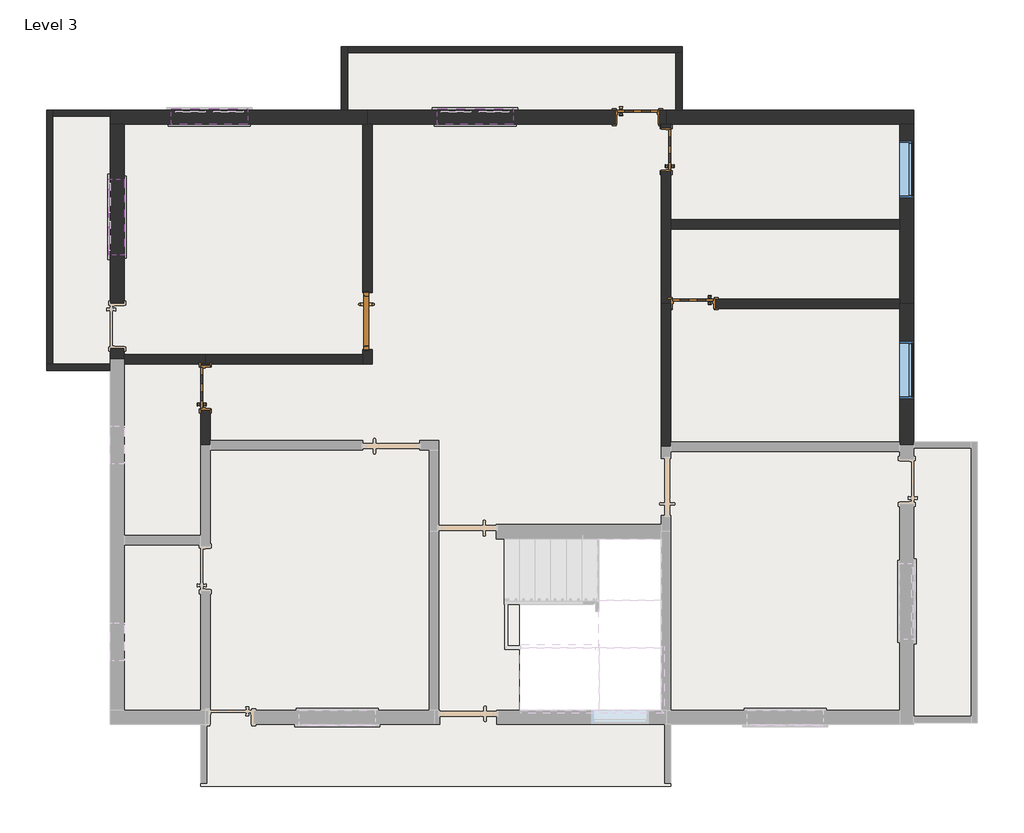
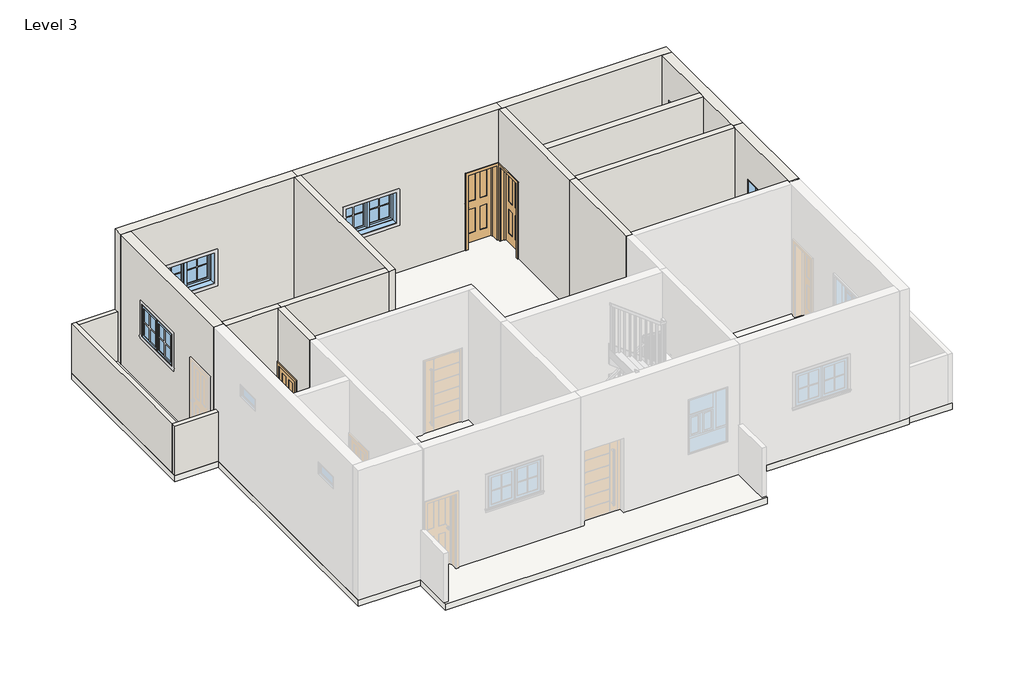
# One storey, part 2 of 3: 20 walls, 5 doors, 5 windows, 1 slab.
"""IFC4 building model written with IfcOpenShell, lengths in millimetres."""

from ifc_helpers import new_model, si_unit, frame, origin, place, context, project, spatial, polyline, outline, extrude, faceted_brep, transform, mapped, element, save
from components import door_3_44036f4b, door_a03dd1d4, door_7109d6db, door_46909e31, m_window_awning_double_horizontal_4_8afcb0b2, m_window_casement_double_sash_variable_3_661e274a

model = new_model("IFC4")

# Units and contexts
model_context = context("Model", 3, world=origin())
ifc_project = project(units=[si_unit("LENGTHUNIT", "METRE", prefix="MILLI")], contexts=[model_context])

# Site, building, storey
site = spatial("IfcSite", under=ifc_project)
building = spatial("IfcBuilding", under=site)
storey = spatial("IfcBuildingStorey", under=building, Name="Level 3", Elevation=6400.8)

# Doors
placement = place(None, origin())
door_3_shape = door_3_44036f4b(model_context)
element("IfcDoor", 1, ObjectType="3'", at=placement, inside=storey, context=model_context, shape_type="MappedRepresentation", body=[
    mapped(door_3_shape, transform((-14176.5794909, 1971.8381491, 6400.8), x_axis=(0.0, -1.0, 0.0), y_axis=(1.0, 0.0, 0.0), z_axis=(0.0, 0.0, 1.0))),
])
door_shape = door_a03dd1d4(model_context)
element("IfcDoor", 2, ObjectType="M_Door-Interior-Single-4_Panel-Wood : 2'2\"", at=placement, inside=storey, context=model_context, shape_type="MappedRepresentation", body=[
    mapped(door_shape, transform((-16770.5544909, 905.4381491, 6400.8), x_axis=(0.0, 1.0, 0.0), y_axis=(-1.0, 0.0, 0.0), z_axis=(0.0, 0.0, 1.0))),
])
door_2_shape = door_7109d6db(model_context)
element("IfcDoor", 3, ObjectType="M_Door-Interior-Single-4_Panel-Wood : 2'2\"", at=placement, inside=storey, context=model_context, shape_type="MappedRepresentation", body=[
    mapped(door_2_shape, transform((-9398.2044909, 4715.4381491, 6400.8), x_axis=(0.0, 1.0, 0.0), y_axis=(-1.0, 0.0, 0.0), z_axis=(0.0, 0.0, 1.0))),
])
element("IfcDoor", 4, ObjectType="M_Door-Interior-Single-4_Panel-Wood : 2'2\"", at=placement, inside=storey, context=model_context, shape_type="MappedRepresentation", body=[
    mapped(door_2_shape, transform((-8969.9794909, 2254.4131491, 6400.8), x_axis=(-1.0, 0.0, 0.0), y_axis=(0.0, -1.0, 0.0), z_axis=(0.0, 0.0, 1.0))),
])
door_4_shape = door_46909e31(model_context)
element("IfcDoor", 5, ObjectType="M_Door-Interior-Single-4_Panel-Wood : 2'2\"", at=placement, inside=storey, context=model_context, shape_type="MappedRepresentation", body=[
    mapped(door_4_shape, transform((-9858.1794909, 5238.9131491, 6400.8), x_axis=(1.0, 0.0, 0.0), y_axis=(0.0, 1.0, 0.0), z_axis=(0.0, 0.0, 1.0))),
])

# Slab
element("IfcSlab", 6, ObjectType="Generic 150mm", at=placement, inside=storey, context=model_context, shape_type="SweptSolid", body=[
    extrude(outline(polyline([(-18291.3794909, 1184.4381491), (-19307.3794909, 1184.4381491), (-19307.3794909, 5350.0381491), (-14596.2721539, 5350.0381491), (-14596.2721539, 6366.0381491), (-9142.3367869, 6366.0381491), (-9142.3367869, 5350.0381491), (-5438.9794909, 5350.0381491), (-5438.9794909, 41.4381491), (-4422.9794909, 41.4381491), (-4422.9794909, -4454.3618509), (-5438.9794909, -4454.3618509), (-5438.9794909, -4479.7618509), (-9325.1794909, -4479.7618509), (-9325.1794909, -5470.3618509), (-16843.5794909, -5470.3618509), (-16843.5794909, -4479.7618509), (-18291.3794909, -4479.7618509), (-18291.3794909, 1184.4381491)]), holes=[polyline([(-11738.1794909, -1507.9618509), (-11738.1794909, -4251.1618509), (-9477.5794909, -4251.1618509), (-9477.5794909, -1507.9618509), (-11738.1794909, -1507.9618509)])]), frame((0.0, 0.0, 6250.8), z_axis=(0.0, 0.0, 1.0), x_axis=(1.0, 0.0, 0.0)), (0.0, 0.0, 1.0), 150.0),
])

# Walls
element("IfcWall", 7, ObjectType="Generic - 4\"", at=placement, inside=storey, context=model_context, shape_type="Brep", body=[
    faceted_brep([(-14494.6721539, 5350.0381491, 6400.8), (-14494.6721539, 6264.4381491, 6400.8), (-14494.6721539, 6366.0381491, 6400.8), (-14494.6721539, 6366.0381491, 7620.0), (-14494.6721539, 6264.4381491, 7620.0), (-14494.6721539, 5350.0381491, 7620.0), (-14596.2721539, 5350.0381491, 6400.8), (-14596.2721539, 5350.0381491, 7620.0), (-14596.2721539, 6366.0381491, 7620.0), (-14596.2721539, 6366.0381491, 6400.8)], [[[0, 1, 2, 3, 4, 5]], [[6, 7, 8, 9]], [[2, 1, 0, 6, 9]], [[5, 4, 3, 8, 7]], [[0, 5, 7, 6]], [[3, 2, 9, 8]]]),
])
element("IfcWall", 8, ObjectType="Generic - 4\"", at=placement, inside=storey, context=model_context, shape_type="Brep", body=[
    faceted_brep([(-14494.6721539, 6264.4381491, 6400.8), (-9243.9367869, 6264.4381491, 6400.8), (-9142.3367869, 6264.4381491, 6400.8), (-9142.3367869, 6264.4381491, 7620.0), (-9243.9367869, 6264.4381491, 7620.0), (-14494.6721539, 6264.4381491, 7620.0), (-14494.6721539, 6366.0381491, 6400.8), (-14494.6721539, 6366.0381491, 7620.0), (-9142.3367869, 6366.0381491, 7620.0), (-9142.3367869, 6366.0381491, 6400.8)], [[[0, 1, 2, 3, 4, 5]], [[6, 7, 8, 9]], [[2, 1, 0, 6, 9]], [[5, 4, 3, 8, 7]], [[0, 5, 7, 6]], [[3, 2, 9, 8]]]),
])
element("IfcWall", 9, ObjectType="Generic - 4\"", at=placement, inside=storey, context=model_context, shape_type="SweptSolid", body=[
    extrude(outline(polyline([(-9243.9367869, 5350.0381491), (-9243.9367869, 6264.4381491), (-9142.3367869, 6264.4381491), (-9142.3367869, 5350.0381491), (-9243.9367869, 5350.0381491)])), frame((0.0, 0.0, 6400.8), z_axis=(0.0, 0.0, 1.0), x_axis=(1.0, 0.0, 0.0)), (0.0, 0.0, 1.0), 1219.2),
])
element("IfcWall", 10, ObjectType="Generic - 4\"", at=placement, inside=storey, context=model_context, shape_type="Brep", body=[
    faceted_brep([(-19307.3794909, 1184.4381491, 6400.8), (-18291.3794909, 1184.4381491, 6400.8), (-18291.3794909, 1184.4381491, 7620.0), (-19307.3794909, 1184.4381491, 7620.0), (-19307.3794909, 1286.0381491, 6400.8), (-19307.3794909, 1286.0381491, 7620.0), (-19205.7794909, 1286.0381491, 7620.0), (-18291.3794909, 1286.0381491, 7620.0), (-18291.3794909, 1286.0381491, 6400.8), (-19205.7794909, 1286.0381491, 6400.8)], [[[0, 1, 2, 3]], [[4, 5, 6, 7, 8, 9]], [[1, 0, 4, 9, 8]], [[3, 2, 7, 6, 5]], [[2, 1, 8, 7]], [[0, 3, 5, 4]]]),
])
element("IfcWall", 11, ObjectType="Generic - 4\"", at=placement, inside=storey, context=model_context, shape_type="Brep", body=[
    faceted_brep([(-19307.3794909, 5350.0381491, 6400.8), (-19307.3794909, 1286.0381491, 6400.8), (-19307.3794909, 1286.0381491, 7620.0), (-19307.3794909, 5350.0381491, 7620.0), (-19205.7794909, 5350.0381491, 6400.8), (-19205.7794909, 5350.0381491, 7620.0), (-19205.7794909, 5248.4381491, 7620.0), (-19205.7794909, 1286.0381491, 7620.0), (-19205.7794909, 1286.0381491, 6400.8), (-19205.7794909, 5248.4381491, 6400.8)], [[[0, 1, 2, 3]], [[4, 5, 6, 7, 8, 9]], [[1, 0, 4, 9, 8]], [[3, 2, 7, 6, 5]], [[2, 1, 8, 7]], [[0, 3, 5, 4]]]),
])
element("IfcWall", 12, ObjectType="Generic - 4\"", at=placement, inside=storey, context=model_context, shape_type="SweptSolid", body=[
    extrude(outline(polyline([(-19205.7794909, 5350.0381491), (-18291.3794909, 5350.0381491), (-18291.3794909, 5248.4381491), (-19205.7794909, 5248.4381491), (-19205.7794909, 5350.0381491)])), frame((0.0, 0.0, 6400.8), z_axis=(0.0, 0.0, 1.0), x_axis=(1.0, 0.0, 0.0)), (0.0, 0.0, 1.0), 1219.2),
])
element("IfcWall", 13, ObjectType="Generic - 6\"", at=placement, inside=storey, context=model_context, shape_type="Brep", body=[
    faceted_brep([(-14252.7794909, 1286.0381491, 9601.2), (-14252.7794909, 1438.4381491, 9601.2), (-14252.7794909, 5121.4381491, 9601.2), (-14252.7794909, 5121.4381491, 6400.8), (-14252.7794909, 2429.0381491, 6400.8), (-14252.7794909, 2429.0381491, 8229.6), (-14252.7794909, 1514.6381491, 8229.6), (-14252.7794909, 1514.6381491, 6400.8), (-14252.7794909, 1438.4381491, 6400.8), (-14252.7794909, 1286.0381491, 6400.8), (-14100.3794909, 5121.4381491, 9601.2), (-14100.3794909, 1286.0381491, 9601.2), (-14100.3794909, 1286.0381491, 6400.8), (-14100.3794909, 1514.6381491, 6400.8), (-14100.3794909, 1514.6381491, 8229.6), (-14100.3794909, 2429.0381491, 8229.6), (-14100.3794909, 2429.0381491, 6400.8), (-14100.3794909, 5121.4381491, 6400.8), (-14232.7794909, 1514.6381491, 6400.8), (-14232.7794909, 1499.6381491, 6400.8), (-14155.7794909, 1499.6381491, 6400.8), (-14155.7794909, 1514.6381491, 6400.8), (-14176.5794909, 5121.4381491, 6400.8), (-14155.7794909, 2429.0381491, 6400.8), (-14155.7794909, 2444.0381491, 6400.8), (-14232.7794909, 2444.0381491, 6400.8), (-14232.7794909, 2429.0381491, 6400.8), (-14176.5794909, 5121.4381491, 9601.2), (-14232.7794909, 2429.0381491, 8229.6), (-14232.7794909, 1514.6381491, 8229.6), (-14155.7794909, 1514.6381491, 8229.6), (-14155.7794909, 2429.0381491, 8229.6), (-14232.7794909, 2444.0381491, 8244.6), (-14155.7794909, 2444.0381491, 8244.6), (-14155.7794909, 1499.6381491, 8244.6), (-14232.7794909, 1499.6381491, 8244.6)], [[[0, 1, 2, 3, 4, 5, 6, 7, 8, 9]], [[10, 11, 12, 13, 14, 15, 16, 17]], [[12, 9, 8, 7, 18, 19, 20, 21, 13]], [[3, 22, 17, 16, 23, 24, 25, 26, 4]], [[2, 1, 0, 11, 10, 27]], [[3, 2, 27, 10, 17, 22]], [[0, 9, 12, 11]], [[5, 28, 29, 6]], [[14, 30, 31, 15]], [[6, 29, 18, 7]], [[30, 14, 13, 21]], [[28, 5, 4, 26]], [[15, 31, 23, 16]], [[32, 33, 34, 35]], [[35, 34, 20, 19]], [[31, 30, 21, 20, 34, 33, 24, 23]], [[33, 32, 25, 24]], [[29, 28, 26, 25, 32, 35, 19, 18]]]),
])
element("IfcWall", 14, ObjectType="Generic - 6\"", at=placement, inside=storey, context=model_context, shape_type="Brep", body=[
    faceted_brep([(-14252.7794909, 1438.4381491, 6400.8), (-16767.3794909, 1438.4381491, 6400.8), (-16767.3794909, 1438.4381491, 9601.2), (-14252.7794909, 1438.4381491, 9601.2), (-14252.7794909, 1286.0381491, 6400.8), (-14252.7794909, 1286.0381491, 9601.2), (-16691.1794909, 1286.0381491, 9601.2), (-16767.3794909, 1286.0381491, 9601.2), (-16767.3794909, 1286.0381491, 6400.8), (-16691.1794909, 1286.0381491, 6400.8)], [[[0, 1, 2, 3]], [[4, 5, 6, 7, 8, 9]], [[1, 0, 4, 9, 8]], [[2, 1, 8, 7]], [[3, 2, 7, 6, 5]], [[0, 3, 5, 4]]]),
])
element("IfcWall", 15, ObjectType="Generic - 6\"", at=placement, inside=storey, context=model_context, shape_type="SweptSolid", body=[
    extrude(outline(polyline([(-5667.5794909, 3445.0381491), (-9325.1794909, 3445.0381491), (-9325.1794909, 3597.4381491), (-5667.5794909, 3597.4381491), (-5667.5794909, 3445.0381491)])), frame((0.0, 0.0, 6400.8), z_axis=(0.0, 0.0, 1.0), x_axis=(1.0, 0.0, 0.0)), (0.0, 0.0, 1.0), 3200.4),
])
element("IfcWall", 16, ObjectType="Generic - 6\"", at=placement, inside=storey, context=model_context, shape_type="Brep", body=[
    faceted_brep([(-9325.1794909, 2327.4381491, 9601.2), (-5667.5794909, 2327.4381491, 9601.2), (-5667.5794909, 2327.4381491, 6400.8), (-8614.7794909, 2327.4381491, 6400.8), (-8614.7794909, 2327.4381491, 8254.6), (-9325.1794909, 2327.4381491, 8254.6), (-5667.5794909, 2175.0381491, 9601.2), (-9325.1794909, 2175.0381491, 9601.2), (-9325.1794909, 2175.0381491, 8254.6), (-8614.7794909, 2175.0381491, 8254.6), (-8614.7794909, 2175.0381491, 6400.8), (-5667.5794909, 2175.0381491, 6400.8), (-5667.5794909, 2251.2381491, 6400.8), (-9325.1794909, 2251.2381491, 9601.2), (-5667.5794909, 2251.2381491, 9601.2)], [[[0, 1, 2, 3, 4, 5]], [[6, 7, 8, 9, 10, 11]], [[2, 12, 11, 10, 3]], [[1, 0, 13, 7, 6, 14]], [[2, 1, 14, 6, 11, 12]], [[7, 13, 0, 5, 8]], [[4, 9, 8, 5]], [[9, 4, 3, 10]]]),
])
element("IfcWall", 17, ObjectType="Generic - 6\"", at=placement, inside=storey, context=model_context, shape_type="Brep", body=[
    faceted_brep([(-9325.1794909, 5121.4381491, 9601.2), (-9325.1794909, 3597.4381491, 9601.2), (-9325.1794909, 3445.0381491, 9601.2), (-9325.1794909, 2327.4381491, 9601.2), (-9325.1794909, 2251.2381491, 9601.2), (-9325.1794909, 2251.2381491, 6400.8), (-9325.1794909, 3445.0381491, 6400.8), (-9325.1794909, 3597.4381491, 6400.8), (-9325.1794909, 4360.2381491, 6400.8), (-9325.1794909, 4360.2381491, 8254.6), (-9325.1794909, 5070.6381491, 8254.6), (-9325.1794909, 5070.6381491, 6400.8), (-9325.1794909, 5121.4381491, 6400.8), (-9477.5794909, 2251.2381491, 9601.2), (-9477.5794909, 5121.4381491, 9601.2), (-9477.5794909, 5121.4381491, 6400.8), (-9477.5794909, 5070.6381491, 6400.8), (-9477.5794909, 5070.6381491, 8254.6), (-9477.5794909, 4360.2381491, 8254.6), (-9477.5794909, 4360.2381491, 6400.8), (-9477.5794909, 2251.2381491, 6400.8), (-9401.3794909, 5121.4381491, 6400.8), (-9401.3794909, 5121.4381491, 9601.2)], [[[0, 1, 2, 3, 4, 5, 6, 7, 8, 9, 10, 11, 12]], [[13, 14, 15, 16, 17, 18, 19, 20]], [[15, 21, 12, 11, 16]], [[5, 20, 19, 8, 7, 6]], [[4, 3, 2, 1, 0, 22, 14, 13]], [[5, 4, 13, 20]], [[0, 12, 21, 15, 14, 22]], [[10, 17, 16, 11]], [[17, 10, 9, 18]], [[18, 9, 8, 19]]]),
])
element("IfcWall", 18, ObjectType="Generic - 6\"", at=placement, inside=storey, context=model_context, shape_type="Brep", body=[
    faceted_brep([(-9325.1794909, -34.7618509, 6400.8), (-9325.1794909, 41.4381491, 6400.8), (-9325.1794909, 2251.2381491, 6400.8), (-9325.1794909, 2251.2381491, 9601.2), (-9325.1794909, 2175.0381491, 9601.2), (-9325.1794909, 41.4381491, 9601.2), (-9325.1794909, -34.7618509, 9601.2), (-9477.5794909, -34.7618509, 6400.8), (-9477.5794909, -34.7618509, 9601.2), (-9477.5794909, 2251.2381491, 9601.2), (-9477.5794909, 2251.2381491, 6400.8)], [[[0, 1, 2, 3, 4, 5, 6]], [[7, 8, 9, 10]], [[2, 1, 0, 7, 10]], [[3, 2, 10, 9]], [[6, 5, 4, 3, 9, 8]], [[0, 6, 8, 7]]]),
])
element("IfcWall", 19, ObjectType="Generic - 6\"", at=placement, inside=storey, context=model_context, shape_type="Brep", body=[
    faceted_brep([(-16691.1794909, 1286.0381491, 9601.2), (-16691.1794909, 66.8381491, 9601.2), (-16691.1794909, -9.3618509, 9601.2), (-16691.1794909, -9.3618509, 6400.8), (-16691.1794909, 66.8381491, 6400.8), (-16691.1794909, 550.2381491, 6400.8), (-16691.1794909, 550.2381491, 8254.6), (-16691.1794909, 1260.6381491, 8254.6), (-16691.1794909, 1260.6381491, 6400.8), (-16691.1794909, 1286.0381491, 6400.8), (-16843.5794909, -9.3618509, 9601.2), (-16843.5794909, 1286.0381491, 9601.2), (-16843.5794909, 1286.0381491, 6400.8), (-16843.5794909, 1260.6381491, 6400.8), (-16843.5794909, 1260.6381491, 8254.6), (-16843.5794909, 550.2381491, 8254.6), (-16843.5794909, 550.2381491, 6400.8), (-16843.5794909, -9.3618509, 6400.8), (-16767.3794909, 1286.0381491, 6400.8), (-16767.3794909, 1286.0381491, 9601.2)], [[[0, 1, 2, 3, 4, 5, 6, 7, 8, 9]], [[10, 11, 12, 13, 14, 15, 16, 17]], [[12, 18, 9, 8, 13]], [[3, 17, 16, 5, 4]], [[2, 1, 0, 19, 11, 10]], [[3, 2, 10, 17]], [[0, 9, 18, 12, 11, 19]], [[7, 14, 13, 8]], [[14, 7, 6, 15]], [[15, 6, 5, 16]]]),
])
element("IfcWall", 20, ObjectType="Generic - 6\"", at=placement, inside=storey, context=model_context, shape_type="Brep", body=[
    faceted_brep([(-16767.3794909, 1438.4381491, 6400.8), (-18062.7794909, 1438.4381491, 6400.8), (-18062.7794909, 1438.4381491, 9601.2), (-16767.3794909, 1438.4381491, 9601.2), (-16767.3794909, 1286.0381491, 6400.8), (-16767.3794909, 1286.0381491, 9601.2), (-16843.5794909, 1286.0381491, 9601.2), (-18062.7794909, 1286.0381491, 9601.2), (-18062.7794909, 1286.0381491, 6400.8), (-16843.5794909, 1286.0381491, 6400.8), (-18062.7794909, 1362.2381491, 6400.8), (-18062.7794909, 1362.2381491, 9601.2)], [[[0, 1, 2, 3]], [[4, 5, 6, 7, 8, 9]], [[1, 0, 4, 9, 8, 10]], [[3, 2, 11, 7, 6, 5]], [[0, 3, 5, 4]], [[2, 1, 10, 8, 7, 11]]]),
])
element("IfcWall", 21, ObjectType="Generic - 9\"", at=placement, inside=storey, context=model_context, shape_type="Brep", body=[
    faceted_brep([(-18291.3794909, 5121.4381491, 9601.2), (-18291.3794909, 5121.4381491, 6400.8), (-18062.7794909, 5121.4381491, 6400.8), (-14252.7794909, 5121.4381491, 6400.8), (-14176.5794909, 5121.4381491, 6400.8), (-14176.5794909, 5121.4381491, 9601.2), (-14252.7794909, 5121.4381491, 9601.2), (-18062.7794909, 5121.4381491, 9601.2), (-16094.2794909, 5121.4381491, 8420.0), (-16094.2794909, 5121.4381491, 7620.0), (-17313.4794909, 5121.4381491, 7620.0), (-17313.4794909, 5121.4381491, 8420.0), (-18291.3794909, 5350.0381491, 6400.8), (-18291.3794909, 5350.0381491, 9601.2), (-14176.5794909, 5350.0381491, 9601.2), (-14176.5794909, 5350.0381491, 6400.8), (-14494.6721539, 5350.0381491, 6400.8), (-14596.2721539, 5350.0381491, 6400.8), (-16094.2794909, 5350.0381491, 8420.0), (-17313.4794909, 5350.0381491, 8420.0), (-17313.4794909, 5350.0381491, 7620.0), (-16094.2794909, 5350.0381491, 7620.0), (-18291.3794909, 5248.4381491, 6400.8)], [[[0, 1, 2, 3, 4, 5, 6, 7], [8, 9, 10, 11]], [[12, 13, 14, 15, 16, 17], [18, 19, 20, 21]], [[4, 3, 2, 1, 22, 12, 17, 16, 15]], [[5, 4, 15, 14]], [[0, 7, 6, 5, 14, 13]], [[0, 13, 12, 22, 1]], [[9, 8, 18, 21]], [[10, 9, 21, 20]], [[11, 10, 20, 19]], [[8, 11, 19, 18]]]),
])
element("IfcWall", 22, ObjectType="Generic - 9\"", at=placement, inside=storey, context=model_context, shape_type="Brep", body=[
    faceted_brep([(-5667.5794909, 5121.4381491, 6400.8), (-5667.5794909, 3597.4381491, 6400.8), (-5667.5794909, 3445.0381491, 6400.8), (-5667.5794909, 2327.4381491, 6400.8), (-5667.5794909, 2251.2381491, 6400.8), (-5667.5794909, 2251.2381491, 9601.2), (-5667.5794909, 2327.4381491, 9601.2), (-5667.5794909, 3445.0381491, 9601.2), (-5667.5794909, 3597.4381491, 9601.2), (-5667.5794909, 5121.4381491, 9601.2), (-5667.5794909, 3943.5131491, 8650.8), (-5667.5794909, 3943.5131491, 7300.8), (-5667.5794909, 4857.9131491, 7300.8), (-5667.5794909, 4857.9131491, 8650.8), (-5438.9794909, 5121.4381491, 6400.8), (-5438.9794909, 5121.4381491, 9601.2), (-5438.9794909, 2251.2381491, 9601.2), (-5438.9794909, 2251.2381491, 6400.8), (-5438.9794909, 3943.5131491, 8650.8), (-5438.9794909, 4857.9131491, 8650.8), (-5438.9794909, 4857.9131491, 7300.8), (-5438.9794909, 3943.5131491, 7300.8)], [[[0, 1, 2, 3, 4, 5, 6, 7, 8, 9], [10, 11, 12, 13]], [[14, 15, 16, 17], [18, 19, 20, 21]], [[4, 3, 2, 1, 0, 14, 17]], [[5, 4, 17, 16]], [[9, 8, 7, 6, 5, 16, 15]], [[0, 9, 15, 14]], [[11, 10, 18, 21]], [[12, 11, 21, 20]], [[13, 12, 20, 19]], [[10, 13, 19, 18]]]),
])
element("IfcWall", 23, ObjectType="Generic - 9\"", at=placement, inside=storey, context=model_context, shape_type="Brep", body=[
    faceted_brep([(-9401.3794909, 5121.4381491, 6400.8), (-9401.3794909, 5121.4381491, 9601.2), (-9477.5794909, 5121.4381491, 9601.2), (-14100.3794909, 5121.4381491, 9601.2), (-14176.5794909, 5121.4381491, 9601.2), (-14176.5794909, 5121.4381491, 6400.8), (-14100.3794909, 5121.4381491, 6400.8), (-10213.3794909, 5121.4381491, 6400.8), (-10213.3794909, 5121.4381491, 8254.6), (-9502.9794909, 5121.4381491, 8254.6), (-9502.9794909, 5121.4381491, 6400.8), (-9477.5794909, 5121.4381491, 6400.8), (-11844.5419909, 5121.4381491, 8420.0), (-11844.5419909, 5121.4381491, 7620.0), (-13063.7419909, 5121.4381491, 7620.0), (-13063.7419909, 5121.4381491, 8420.0), (-9401.3794909, 5350.0381491, 9601.2), (-9401.3794909, 5350.0381491, 6400.8), (-9502.9794909, 5350.0381491, 6400.8), (-9502.9794909, 5350.0381491, 8254.6), (-10213.3794909, 5350.0381491, 8254.6), (-10213.3794909, 5350.0381491, 6400.8), (-14176.5794909, 5350.0381491, 6400.8), (-14176.5794909, 5350.0381491, 9601.2), (-11844.5419909, 5350.0381491, 8420.0), (-13063.7419909, 5350.0381491, 8420.0), (-13063.7419909, 5350.0381491, 7620.0), (-11844.5419909, 5350.0381491, 7620.0)], [[[0, 1, 2, 3, 4, 5, 6, 7, 8, 9, 10, 11], [12, 13, 14, 15]], [[16, 17, 18, 19, 20, 21, 22, 23], [24, 25, 26, 27]], [[5, 22, 21, 7, 6]], [[17, 0, 11, 10, 18]], [[1, 0, 17, 16]], [[4, 3, 2, 1, 16, 23]], [[5, 4, 23, 22]], [[12, 15, 25, 24]], [[15, 14, 26, 25]], [[14, 13, 27, 26]], [[13, 12, 24, 27]], [[9, 19, 18, 10]], [[19, 9, 8, 20]], [[20, 8, 7, 21]]]),
])
element("IfcWall", 24, ObjectType="Generic - 9\"", at=placement, inside=storey, context=model_context, shape_type="Brep", body=[
    faceted_brep([(-9401.3794909, 5121.4381491, 6400.8), (-9325.1794909, 5121.4381491, 6400.8), (-5667.5794909, 5121.4381491, 6400.8), (-5438.9794909, 5121.4381491, 6400.8), (-5438.9794909, 5121.4381491, 9601.2), (-5667.5794909, 5121.4381491, 9601.2), (-9325.1794909, 5121.4381491, 9601.2), (-9401.3794909, 5121.4381491, 9601.2), (-9401.3794909, 5350.0381491, 6400.8), (-9401.3794909, 5350.0381491, 9601.2), (-5438.9794909, 5350.0381491, 9601.2), (-5438.9794909, 5350.0381491, 6400.8), (-9142.3367869, 5350.0381491, 6400.8), (-9243.9367869, 5350.0381491, 6400.8)], [[[0, 1, 2, 3, 4, 5, 6, 7]], [[8, 9, 10, 11, 12, 13]], [[3, 2, 1, 0, 8, 13, 12, 11]], [[7, 6, 5, 4, 10, 9]], [[0, 7, 9, 8]], [[4, 3, 11, 10]]]),
])
element("IfcWall", 25, ObjectType="Generic - 9\"", at=placement, inside=storey, context=model_context, shape_type="Brep", body=[
    faceted_brep([(-5667.5794909, 2251.2381491, 6400.8), (-5667.5794909, 2175.0381491, 6400.8), (-5667.5794909, 41.4381491, 6400.8), (-5667.5794909, -34.7618509, 6400.8), (-5667.5794909, -34.7618509, 9601.2), (-5667.5794909, 41.4381491, 9601.2), (-5667.5794909, 2175.0381491, 9601.2), (-5667.5794909, 2251.2381491, 9601.2), (-5667.5794909, 732.0006491, 8650.8), (-5667.5794909, 732.0006491, 7300.8), (-5667.5794909, 1646.4006491, 7300.8), (-5667.5794909, 1646.4006491, 8650.8), (-5438.9794909, 2251.2381491, 6400.8), (-5438.9794909, 2251.2381491, 9601.2), (-5438.9794909, -34.7618509, 9601.2), (-5438.9794909, -34.7618509, 6400.8), (-5438.9794909, 41.4381491, 6400.8), (-5438.9794909, 732.0006491, 8650.8), (-5438.9794909, 1646.4006491, 8650.8), (-5438.9794909, 1646.4006491, 7300.8), (-5438.9794909, 732.0006491, 7300.8)], [[[0, 1, 2, 3, 4, 5, 6, 7], [8, 9, 10, 11]], [[12, 13, 14, 15, 16], [17, 18, 19, 20]], [[3, 2, 1, 0, 12, 16, 15]], [[7, 6, 5, 4, 14, 13]], [[0, 7, 13, 12]], [[8, 11, 18, 17]], [[11, 10, 19, 18]], [[10, 9, 20, 19]], [[9, 8, 17, 20]], [[3, 15, 14, 4]]]),
])
element("IfcWall", 26, ObjectType="Generic - 9\"", at=placement, inside=storey, context=model_context, shape_type="Brep", body=[
    faceted_brep([(-18062.7794909, 5121.4381491, 9601.2), (-18062.7794909, 1438.4381491, 9601.2), (-18062.7794909, 1362.2381491, 9601.2), (-18062.7794909, 1362.2381491, 6400.8), (-18062.7794909, 1438.4381491, 6400.8), (-18062.7794909, 1540.0381491, 6400.8), (-18062.7794909, 1540.0381491, 8254.6), (-18062.7794909, 2250.4381491, 8254.6), (-18062.7794909, 2250.4381491, 6400.8), (-18062.7794909, 5121.4381491, 6400.8), (-18062.7794909, 4247.5131491, 8420.0), (-18062.7794909, 4247.5131491, 7620.0), (-18062.7794909, 3028.3131491, 7620.0), (-18062.7794909, 3028.3131491, 8420.0), (-18291.3794909, 1362.2381491, 9601.2), (-18291.3794909, 5121.4381491, 9601.2), (-18291.3794909, 5121.4381491, 6400.8), (-18291.3794909, 2250.4381491, 6400.8), (-18291.3794909, 2250.4381491, 8254.6), (-18291.3794909, 1540.0381491, 8254.6), (-18291.3794909, 1540.0381491, 6400.8), (-18291.3794909, 1362.2381491, 6400.8), (-18291.3794909, 4247.5131491, 8420.0), (-18291.3794909, 3028.3131491, 8420.0), (-18291.3794909, 3028.3131491, 7620.0), (-18291.3794909, 4247.5131491, 7620.0)], [[[0, 1, 2, 3, 4, 5, 6, 7, 8, 9], [10, 11, 12, 13]], [[14, 15, 16, 17, 18, 19, 20, 21], [22, 23, 24, 25]], [[16, 9, 8, 17]], [[3, 21, 20, 5, 4]], [[2, 1, 0, 15, 14]], [[9, 16, 15, 0]], [[10, 13, 23, 22]], [[13, 12, 24, 23]], [[12, 11, 25, 24]], [[11, 10, 22, 25]], [[19, 6, 5, 20]], [[6, 19, 18, 7]], [[7, 18, 17, 8]], [[2, 14, 21, 3]]]),
])

# Windows
m_window_awning_double_horizontal_4_shape = m_window_awning_double_horizontal_4_8afcb0b2(model_context)
element("IfcWindow", 27, ObjectType="M_Window-Awning-Double-Horizontal : 4'", at=placement, inside=storey, context=model_context, shape_type="MappedRepresentation", body=[
    mapped(m_window_awning_double_horizontal_4_shape, transform((-16703.8794909, 5235.7381491, 6720.0), x_axis=(1.0, 0.0, 0.0), y_axis=(0.0, 1.0, 0.0), z_axis=(0.0, 0.0, 1.0))),
])
element("IfcWindow", 28, ObjectType="M_Window-Awning-Double-Horizontal : 4'", at=placement, inside=storey, context=model_context, shape_type="MappedRepresentation", body=[
    mapped(m_window_awning_double_horizontal_4_shape, transform((-18177.0794909, 3637.9131491, 6720.0), x_axis=(0.0, 1.0, 0.0), y_axis=(-1.0, 0.0, 0.0), z_axis=(0.0, 0.0, 1.0))),
])
element("IfcWindow", 29, ObjectType="M_Window-Awning-Double-Horizontal : 4'", at=placement, inside=storey, context=model_context, shape_type="MappedRepresentation", body=[
    mapped(m_window_awning_double_horizontal_4_shape, transform((-12454.1419909, 5235.7381491, 6720.0), x_axis=(1.0, 0.0, 0.0), y_axis=(0.0, 1.0, 0.0), z_axis=(0.0, 0.0, 1.0))),
])
m_window_casement_double_sash_variable_3_shape = m_window_casement_double_sash_variable_3_661e274a(model_context)
element("IfcWindow", 30, ObjectType="M_Window-Casement-Double-Sash-Variable : 3'", at=placement, inside=storey, context=model_context, shape_type="MappedRepresentation", body=[
    mapped(m_window_casement_double_sash_variable_3_shape, transform((-5553.2794909, 1189.2006491, 6400.8), x_axis=(0.0, -1.0, 0.0), y_axis=(1.0, 0.0, 0.0), z_axis=(0.0, 0.0, 1.0))),
])
element("IfcWindow", 31, ObjectType="M_Window-Casement-Double-Sash-Variable : 3'", at=placement, inside=storey, context=model_context, shape_type="MappedRepresentation", body=[
    mapped(m_window_casement_double_sash_variable_3_shape, transform((-5553.2794909, 4400.7131491, 6400.8), x_axis=(0.0, -1.0, 0.0), y_axis=(1.0, 0.0, 0.0), z_axis=(0.0, 0.0, 1.0))),
])

save(model, "model.ifc")

# Revit data of these elements
# Type "3'"
#   Type Mark = "41"
#   Water resistance = "up to Class E900, EN 12208:2001"
#   Uniclass2015Version = "v1.21"
#   Uniclass2015Reference = "Ss_25_30_20_30"
#   Uniclass2015Description = "Frame and door leaf system"
#   URL = "www.aluprof.com"
#   Type IFC Predefined Type = "USERDEFINED"
#   Right-hand / Left-hand door [instance default] = ""
#   Resistance to wind load = "up to Class C5/B5, EN 12210:2001"
#   Insert type = "ST"
#   Hardware [instance default] = ""
#   Product page = "https://aluprof.com/en/architects/offer/window-and-door-systems/panel-doors#visualisation"
#   Operation = "SinglePanelOutwardOpening"
#   Opening type = "Outward"
#   NBSReference = "25-50-20/125"
#   NBSDescription = "Frame and door leaf system"
#   Important = "The actual acceptable construction dimensions are dependent on the selection of profiles and hardware, glazing type, construction weight and the construction’s operating conditions. These should be determined by a suitably qualified person, and using ALUPROF’s calculation software"
#   IfcExportType = "USERDEFINED"
#   IfcExportAs = "IfcDoorType"
#   Handle type [instance default] = ""
#   Manufacturer = "ALUPROF SA"
#   Export Type to IFC As = "IfcDoorType"
#   Door sill type [instance default] = ""
#   Description = "External single-leaf panel door outward opening"
#   Model = "MB-86 ST Panel Door AD07"
#   Content of the recyclate in the material = "69.2%"
#   COBie.Type.WarrantyDurationParts = ""
#   COBie.Type.Name = ""
#   COBie.Type.Manufacturer = "ALUPROF SA"
#   COBie.Space.Name = ""
#   COBie.Floor.Name = ""
#   COBie.Facility.Name = ""
#   COBie.CreatedOn = ""
#   COBie.Component.WarrantyStartDate = ""
#   COBie.Component.Name = "MB-86 ST Panel Door AD07"
#   Burglar resistance = "RC2"
#   Air permeability = "up to Class 4, EN 12207:2001"
#   Width of the active leaf = 2' - 8.17717"
#   Placement in wall = 0' - 0.7874"
#   Thickness = 0' - 3.0315"
#   Height of the opening sash = 5' - 9.44094"
#   Handle Offset = 3' - 5.33858"
#   Rough Height = 6' - 2.40945"
#   Rough Width = 3' - 1.1811"
#   Height = 6' - 0"
#   Width = 3' - 0"
#   Construction depth = 0' - 3.0315"
#   Clear opening width = 2' - 3.94882"
#   Clear opening height = 5' - 8.47638"
#   Height of the array = 0' - 11.08136"
#   Schedule No. [instance default] = 1
#   Handrail [instance default] = yes
#   IsExternal = yes
#   Handle [instance default] = no
#   Door closer [instance default] = no
#   Function = 1
#   COBie.Type = yes
#   COBie = yes
#   Access control [instance default] = no
#   Panel = element 361060
#   Wall Closure = (empty or 0)
# Type "M_Door-Interior-Single-4_Panel-Wood : 2'2\""
#   Type Mark = "43"
#   Assembly Code = "C1020300"
#   Analytic Construction = "Wooden"
#   Top Rail = 0' - 4.72441"
#   Thickness = 0' - 1.37795"
#   Thermal Resistance (R) = 0.455703 (m²·K)/W
#   Swing Angle [instance default] = 90.00°
#   Stiles = 0' - 4.72441"
#   Rough Width = 2' - 3.9685"
#   Rough Height = 6' - 0.98425"
#   Mullion = 0' - 4.52756"
#   Lock Rail = 0' - 7.87402"
#   Height = 6' - 0"
#   Width = 2' - 2"
#   Heat Transfer Coefficient (U) = 2.19465 W/(m²·K)
#   Bottom Rail = 0' - 9.05512"
#   Trim Material = Cherry
#   Panel Material = Cherry
#   Frame Material = Cherry
#   Door Handle Material = Aluminum
#   Visual Light Transmittance = 0
#   Solar Heat Gain Coefficient = 0
#   Wall Closure = (empty or 0)
#   Function = (empty or 0)
# Type "Generic 150mm"
#   Function = 0
#   Layers, outside or top first: 0' - 5.90551" no material (function 1)
# Type "Generic - 4\""
#   Layers, outside or top first: 0' - 4" no material (function 1)
# Type "Generic - 6\""
#   Layers, outside or top first: 0' - 6" no material (function 1)
# Type "Generic - 9\""
#   Layers, outside or top first: 0' - 9" no material (function 1)
# Type "M_Window-Awning-Double-Horizontal : 4'"
#   Type Mark = "28"
#   Fire Rating = "0.5h"
#   Assembly Code = "B2020100"
#   Analytic Construction = "Double glazing - domestic"
#   Window Inset [instance default] = 0' - 0"
#   Wall Thickness [instance default] = 0' - 5.90551"
#   Interior Wall Closure [instance default] = 0' - 2.15551"
#   Half Width = 2' - 0"
#   Visual Light Transmittance = 0.81
#   Thermal Resistance (R) = 0.319569 (m²·K)/W
#   Solar Heat Gain Coefficient = 0.76
#   Rough Width = 4' - 0.59055"
#   Rough Height = 2' - 8.08661"
#   Height = 2' - 7.49606"
#   Heat Transfer Coefficient (U) = 3.12929 W/(m²·K)
#   Frame Extension [instance default] = 0' - 0 1/4"
#   Exterior Wall Closure [instance default] = 0' - 1 1/4"
#   Extension Jamb [instance default] = 0' - 2.15551"
#   Default Sill Height = 2' - 11.43307"
#   Width = 4' - 0"
#   Muntin Visibility = yes
#   Interior Trim Visibility [instance default] = yes
#   Exterior Trim Visibility [instance default] = yes
#   Extension Jamb Visibility [instance default] = yes
#   Interior Trim Material = Wood - Stained
#   Muntin Pattern = M_Muntin Pattern_2x2 : M_Muntin Pattern_2x2
#   Interior Trim = M_Trim-Window-Interior-Flat : Picture Frame
#   Interior Frame Material = Wood - Stained
#   Glass Panel Material = Glass
#   Exterior Trim Material = Clad - White
#   Exterior Trim = M_Trim-Window-Exterior-Flat : with Sill
#   Exterior Frame Material = Clad - White
#   Wall Closure = (empty or 0)
# Type "M_Window-Casement-Double-Sash-Variable : 3'"
#   Type Mark = "36"
#   Fire Rating = "0.5h"
#   Assembly Code = "B2020100"
#   Analytic Construction = "Double glazing - domestic"
#   Window Inset [instance default] = 0' - 0 5/8"
#   Wall Thickness [instance default] = 0' - 5.90551"
#   Visual Light Transmittance = 0.81
#   Transom Height Ratio = 0.3
#   Transom Height = 1' - 3.94488"
#   Thermal Resistance (R) = 0.319569 (m²·K)/W
#   Solar Heat Gain Coefficient = 0.76
#   Rough Width = 3' - 0.59055"
#   Rough Height = 4' - 5.74016"
#   Opening Window Height = 1' - 9.25984"
#   Heat Transfer Coefficient (U) = 3.12929 W/(m²·K)
#   Height = 4' - 5.14961"
#   Frame Gap 3 [instance default] = 0' - 1.65041"
#   Frame Gap 2 [instance default] = 0' - 0.62598"
#   Frame Gap 1 = 0' - 1 51/128"
#   Window Width = 1' - 0"
#   Default Sill Height = 2' - 11.43307"
#   Width = 3' - 0"
#   Frame Material = Metal - Aluminum
#   Glass Panel Material = Glass
#   Wall Closure = (empty or 0)
# Element 1 (IfcDoor, "3'")
#   Right-hand / Left-hand door = ""
#   Hardware = ""
#   Handle type = ""
#   Door sill type = ""
#   Schedule No. = 1
#   Handrail = yes
#   Handle = no
#   Door closer = no
#   Access control = no
#   Phase Created = New Construction
# Elements 2, 3, 4, 5 (IfcDoor, "M_Door-Interior-Single-4_Panel-Wood : 2'2\"")
#   Swing Angle = 90.00°
#   Phase Created = New Construction
#   Materials on its faces: "Cherry", "Aluminum"
# Element 6 (IfcSlab, "Generic 150mm")
#   Height Offset From Level = 0' - 0"
#   Phase Created = New Construction
#   Materials on its faces: "WALL2", "Default Floor", "FLOORING TILES 1"
# Elements 7, 8, 9, 10 (IfcWall, "Generic - 4\"")
#   Top Offset = 0' - 0"
#   Base Offset = 0' - 0"
#   Unconnected Height = 4' - 0"
#   wall height = 4' - 0"
#   Phase Created = New Construction
#   Base Constraint = Level 3
#   Materials on its faces: "Default Wall", "WALL2"
# Elements 11, 12 (IfcWall, "Generic - 4\"")
#   Top Offset = 0' - 0"
#   Base Offset = 0' - 0"
#   Unconnected Height = 4' - 0"
#   wall height = 4' - 0"
#   Phase Created = New Construction
#   Base Constraint = Level 3
#   Materials on its faces: "WALL2", "Default Wall"
# Element 13 (IfcWall, "Generic - 6\"")
#   Top Offset = 0' - 0"
#   Base Offset = 0' - 0"
#   Unconnected Height = 10' - 6"
#   wall height = 10' - 6"
#   Phase Created = New Construction
#   Base Constraint = Level 3
#   Materials on its faces: "Default Wall", "LIVING 2", "BED ROOM WALL1"
# Element 14 (IfcWall, "Generic - 6\"")
#   Top Offset = 0' - 0"
#   Base Offset = 0' - 0"
#   Unconnected Height = 10' - 6"
#   wall height = 10' - 6"
#   Phase Created = New Construction
#   Base Constraint = Level 3
#   Materials on its faces: "Default Wall", "BED ROOM WALL 2", "LIVING 2"
# Element 15 (IfcWall, "Generic - 6\"")
#   Top Offset = 0' - 0"
#   Base Offset = 0' - 0"
#   Unconnected Height = 10' - 6"
#   wall height = 10' - 6"
#   Phase Created = New Construction
#   Base Constraint = Level 3
#   Materials on its faces: "Default Wall", "BED ROOM WALL 3", "BED ROOM WALL1"
# Elements 16, 17 (IfcWall, "Generic - 6\"")
#   Top Offset = 0' - 0"
#   Base Offset = 0' - 0"
#   Unconnected Height = 10' - 6"
#   wall height = 10' - 6"
#   Phase Created = New Construction
#   Base Constraint = Level 3
#   Materials on its faces: "Default Wall", "BED ROOM WALL1", "LIVING 2"
# Element 18 (IfcWall, "Generic - 6\"")
#   Top Offset = 0' - 0"
#   Base Offset = 0' - 0"
#   Unconnected Height = 10' - 6"
#   wall height = 10' - 6"
#   Phase Created = New Construction
#   Base Constraint = Level 3
#   Materials on its faces: "Default Wall", "LIVING", "LIVING 2"
# Element 19 (IfcWall, "Generic - 6\"")
#   Top Offset = 0' - 0"
#   Base Offset = 0' - 0"
#   Unconnected Height = 10' - 6"
#   wall height = 10' - 6"
#   Phase Created = New Construction
#   Base Constraint = Level 3
#   Materials on its faces: "Default Wall", "LIVING 2", "BATH ROOM WALL 1"
# Element 20 (IfcWall, "Generic - 6\"")
#   Top Offset = 0' - 0"
#   Base Offset = 0' - 0"
#   Unconnected Height = 10' - 6"
#   wall height = 10' - 6"
#   Phase Created = New Construction
#   Base Constraint = Level 3
#   Materials on its faces: "Default Wall", "BED ROOM WALL 2", "BATH ROOM WALL 1"
# Element 21 (IfcWall, "Generic - 9\"")
#   Top Offset = 0' - 0"
#   Base Offset = 0' - 0"
#   Unconnected Height = 10' - 6"
#   wall height = 10' - 6"
#   Phase Created = New Construction
#   Base Constraint = Level 3
#   Materials on its faces: "Default Wall", "WALL2", "BED ROOM WALL1"
# Element 22 (IfcWall, "Generic - 9\"")
#   Top Offset = 0' - 0"
#   Base Offset = 0' - 0"
#   Unconnected Height = 10' - 6"
#   wall height = 10' - 6"
#   Phase Created = New Construction
#   Base Constraint = Level 3
#   Materials on its faces: "Default Wall", "BED ROOM WALL 3", "WALL2"
# Elements 23, 25 (IfcWall, "Generic - 9\"")
#   Top Offset = 0' - 0"
#   Base Offset = 0' - 0"
#   Unconnected Height = 10' - 6"
#   wall height = 10' - 6"
#   Phase Created = New Construction
#   Base Constraint = Level 3
#   Materials on its faces: "Default Wall", "LIVING 2", "WALL2"
# Element 24 (IfcWall, "Generic - 9\"")
#   Top Offset = 0' - 0"
#   Base Offset = 0' - 0"
#   Unconnected Height = 10' - 6"
#   wall height = 10' - 6"
#   Phase Created = New Construction
#   Base Constraint = Level 3
#   Materials on its faces: "Default Wall", "WALL2", "BED ROOM WALL 3"
# Element 26 (IfcWall, "Generic - 9\"")
#   Top Offset = 0' - 0"
#   Base Offset = 0' - 0"
#   Unconnected Height = 10' - 6"
#   wall height = 10' - 6"
#   Phase Created = New Construction
#   Base Constraint = Level 3
#   Materials on its faces: "Default Wall", "BED ROOM WALL 2", "WALL2"
# Element 27 (IfcWindow, "M_Window-Awning-Double-Horizontal : 4'")
#   Mark = "24"
#   Window Inset = 0' - 0"
#   Interior Wall Closure = 0' - 2.15551"
#   Frame Extension = 0' - 0 1/4"
#   Exterior Wall Closure = 0' - 1 1/4"
#   Interior Trim Visibility = yes
#   Exterior Trim Visibility = yes
#   Phase Created = New Construction
#   Materials on its faces: "Wood - Stained", "Glass", "Clad - White"
# Element 28 (IfcWindow, "M_Window-Awning-Double-Horizontal : 4'")
#   Mark = "25"
#   Window Inset = 0' - 0"
#   Interior Wall Closure = 0' - 2.15551"
#   Frame Extension = 0' - 0 1/4"
#   Exterior Wall Closure = 0' - 1 1/4"
#   Interior Trim Visibility = yes
#   Exterior Trim Visibility = yes
#   Phase Created = New Construction
#   Materials on its faces: "Wood - Stained", "Glass", "Clad - White"
# Element 29 (IfcWindow, "M_Window-Awning-Double-Horizontal : 4'")
#   Mark = "26"
#   Window Inset = 0' - 0"
#   Interior Wall Closure = 0' - 2.15551"
#   Frame Extension = 0' - 0 1/4"
#   Exterior Wall Closure = 0' - 1 1/4"
#   Interior Trim Visibility = yes
#   Exterior Trim Visibility = yes
#   Phase Created = New Construction
#   Materials on its faces: "Wood - Stained", "Glass", "Clad - White"
# Element 30 (IfcWindow, "M_Window-Casement-Double-Sash-Variable : 3'")
#   Mark = "30"
#   Window Inset = 0' - 0 5/8"
#   Frame Gap 3 = 0' - 1.65041"
#   Frame Gap 2 = 0' - 0.62598"
#   Phase Created = New Construction
#   Materials on its faces: "Metal - Aluminum", "Glass"
# Element 31 (IfcWindow, "M_Window-Casement-Double-Sash-Variable : 3'")
#   Mark = "31"
#   Window Inset = 0' - 0 5/8"
#   Frame Gap 3 = 0' - 1.65041"
#   Frame Gap 2 = 0' - 0.62598"
#   Phase Created = New Construction
#   Materials on its faces: "Metal - Aluminum", "Glass"
# Materials
#   "Cherry": class "Wood", colour RGB 226 177 128, transparency 0, Description = "Prunus Serotina", Cost = 0
#   "Aluminum": class "Metal", colour RGB 247 247 247, transparency 0, Description = "Aluminum 6061", Cost = 0
#   "Wood - Stained": class "Wood", colour RGB 224 178 126, transparency 0, Cost = 0
#   "Glass": class "Glass", colour RGB 0 128 192, transparency 0.9, Description = "Soda Lime Glass", Cost = 0
#   "Clad - White": class "Wood", colour RGB 242 242 238, transparency 0, Cost = 0
#   "Metal - Aluminum": class "Metal", colour RGB 247 247 247, transparency 0
#   "WALL2": class "Generic", colour RGB 120 120 120, transparency 0, Cost = 0
#   "Default Floor": colour RGB 127 127 127, transparency 0, Cost = 0
#   "FLOORING TILES 1": class "Generic", colour RGB 120 120 120, transparency 0, Cost = 0
#   "Default Wall": colour RGB 128 128 128, transparency 0, Cost = 0
#   "LIVING 2": class "Generic", colour RGB 120 120 120, transparency 0, Cost = 0
#   "BED ROOM WALL1": class "Generic", colour RGB 120 120 120, transparency 0, Cost = 0
#   "BED ROOM WALL 2": class "Generic", colour RGB 120 120 120, transparency 0, Cost = 0
#   "BED ROOM WALL 3": class "Generic", colour RGB 120 120 120, transparency 0, Cost = 0
#   "LIVING": class "Generic", colour RGB 120 120 120, transparency 0, Cost = 0
#   "BATH ROOM WALL 1": class "Generic", colour RGB 120 120 120, transparency 0, Cost = 0
